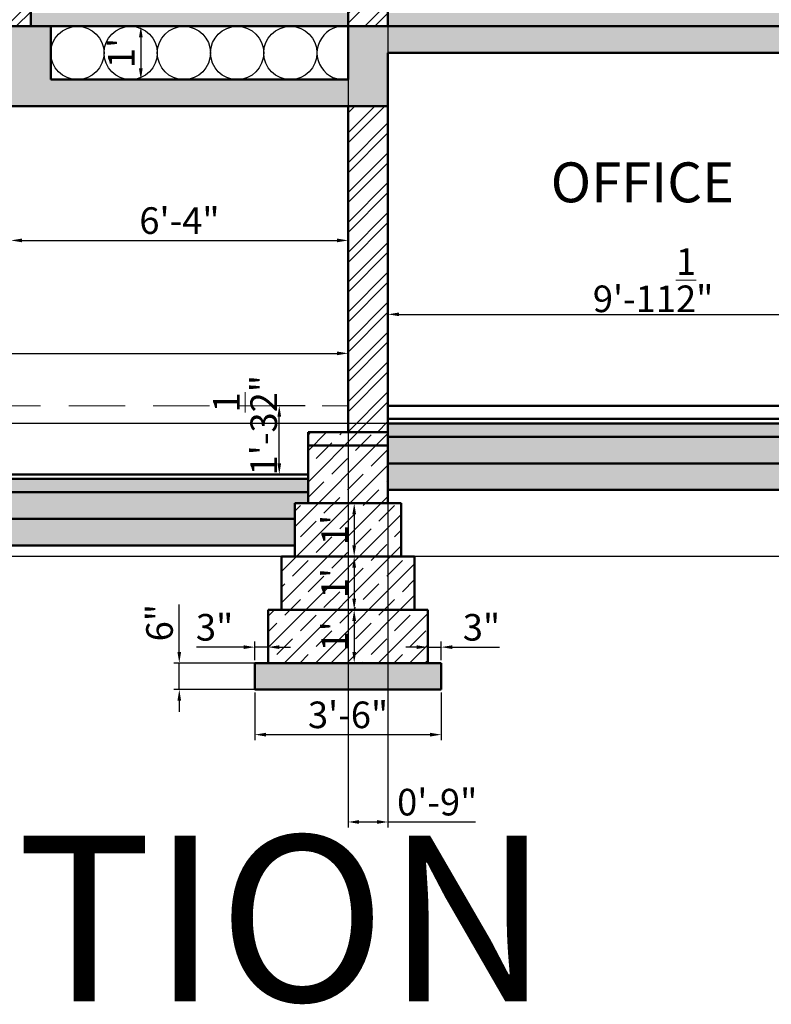
# Model space of a CAD drawing. Units: inches. Extents: x 1615 to 2231, y 1931 to 2519.
# Tile 3 of 6: x 1892 to 2061, y 1931 to 2153. Entities that reach past the tile are written whole.
import ezdxf

# ---------------------------------------------------------------- set-up
doc = ezdxf.new("R2010")
doc.units = ezdxf.units.IN
doc.linetypes.add('DASHED', pattern=[19.05, 12.7, -6.35])
for name, color, linetype, lineweight in [('A-ANNO-DIMS', 2, 'Continuous', 18), ('A-ANNO-TEXT', 7, 'Continuous', 35), ('A-AREA-IDEN', 7, 'Continuous', 25), ('A-SECT', 7, 'Continuous', 50), ('A-SECT-HIDN', 8, 'DASHED', 18), ('A-WALL-PATT', 8, 'Continuous', 13), ('C-TOPO-PATT', 252, 'Continuous', 13), ('S-FNDN', 1, 'Continuous', 50), ('S-FNDN-PATT', 8, 'Continuous', 13), ('S-SLAB', 7, 'Continuous', 25)]:
    doc.layers.add(name, color=color, linetype=linetype, lineweight=lineweight)
doc.styles.get("Standard").update_dxf_attribs({"font": 'arial.ttf'})
doc.dimstyles.new('ISO-25', dxfattribs={"dimtxt": 6, "dimasz": 2.5, "dimexe": 1.25, "dimexo": 0.625, "dimtad": 1, "dimdec": 1, "dimlunit": 4, "dimtxsty": 'Standard', "dimcen": 2.5, "dimadec": 0, "dimazin": 0, "dimtfac": 1, "dimtdec": 1, "dimtmove": 0, "dimatfit": 3, "dimfxl": 1, "dimarcsym": 0})

# ---------------------------------------------------------------- blocks, each defined once
blk = doc.blocks.new('*D9')
at = {"layer": 'A-ANNO-DIMS', "color": 0, "lineweight": -2, "transparency": 16777216}
for p, q in [((1693.37, 2070.69), (1693.37, 2079.07)), ((1695.87, 2077.82), (1963.37, 2077.82)), ((1965.87, 2070.69), (1965.87, 2079.07))]:
    blk.add_line(p, q, dxfattribs=at)
at = {"layer": 'A-ANNO-DIMS', "color": 0, "lineweight": 100, "transparency": 16777216}
for points in [[(1695.87, 2078.24), (1695.87, 2077.4), (1693.37, 2077.82)], [(1963.37, 2078.24), (1963.37, 2077.4), (1965.87, 2077.82)]]:
    blk.add_solid(points, dxfattribs=at)
at = {"layer": 'Defpoints', "color": 0, "lineweight": 100, "transparency": 16777216}
for p in [(1965.87, 2077.82), (1693.37, 2070.06), (1965.87, 2070.06)]:
    blk.add_point(p, dxfattribs=at)
at = {"layer": 'A-ANNO-DIMS', "color": 0, "transparency": 16777216, "insert": (1829.62, 2085.52), "char_height": 6, "attachment_point": 5}
blk.add_mtext('22\'-8{\\H1x;\\S1/2;}"', dxfattribs=at)
blk = doc.blocks.new('*D10')
at = {"layer": 'A-ANNO-DIMS', "color": 0, "lineweight": -2, "transparency": 16777216}
for p, q in [((1956.24, 2066.03), (1949.12, 2066.03)), ((1950.37, 2053.03), (1950.37, 2063.53)), ((1956.24, 2050.53), (1949.12, 2050.53))]:
    blk.add_line(p, q, dxfattribs=at)
at = {"layer": 'A-ANNO-DIMS', "color": 0, "lineweight": 100, "transparency": 16777216}
for points in [[(1949.96, 2063.53), (1950.79, 2063.53), (1950.37, 2066.03)], [(1949.96, 2053.03), (1950.79, 2053.03), (1950.37, 2050.53)]]:
    blk.add_solid(points, dxfattribs=at)
at = {"layer": 'Defpoints', "color": 0, "lineweight": 100, "transparency": 16777216}
for p in [(1950.37, 2066.03), (1956.87, 2066.03), (1956.87, 2050.53)]:
    blk.add_point(p, dxfattribs=at)
at = {"layer": 'A-ANNO-DIMS', "color": 0, "transparency": 16777216, "insert": (1942.67, 2061.63), "char_height": 6, "attachment_point": 5, "rotation": 90}
blk.add_mtext('1\'-3{\\H1x;\\S1/2;}"', dxfattribs=at)
blk = doc.blocks.new('*D17')
at = {"layer": 'A-ANNO-DIMS', "color": 0, "lineweight": -2, "transparency": 16777216}
for p, q in [((1944.87, 2001.4), (1944.87, 1990.63)), ((1986.87, 2001.4), (1986.87, 1990.63)), ((1947.37, 1991.88), (1984.37, 1991.88))]:
    blk.add_line(p, q, dxfattribs=at)
at = {"layer": 'A-ANNO-DIMS', "color": 0, "lineweight": 100, "transparency": 16777216}
for points in [[(1947.37, 1992.3), (1947.37, 1991.46), (1944.87, 1991.88)], [(1984.37, 1992.3), (1984.37, 1991.46), (1986.87, 1991.88)]]:
    blk.add_solid(points, dxfattribs=at)
at = {"layer": 'Defpoints', "color": 0, "lineweight": 100, "transparency": 16777216}
for p in [(1944.87, 2002.03), (1986.87, 2002.03), (1986.87, 1991.88)]:
    blk.add_point(p, dxfattribs=at)
at = {"layer": 'A-ANNO-DIMS', "color": 0, "transparency": 16777216, "insert": (1965.87, 1995.57), "char_height": 6, "attachment_point": 5}
blk.add_mtext('3\'-6"', dxfattribs=at)
blk = doc.blocks.new('*D18')
at = {"layer": 'A-ANNO-DIMS', "color": 0, "lineweight": -2, "transparency": 16777216}
for p, q in [((1983.87, 2008.41), (1983.87, 2012.86)), ((1986.87, 2008.65), (1986.87, 2012.86)), ((1981.37, 2011.61), (1978.87, 2011.61)), ((1983.87, 2011.61), (1986.87, 2011.61)), ((1989.37, 2011.61), (2000.01, 2011.61))]:
    blk.add_line(p, q, dxfattribs=at)
at = {"layer": 'A-ANNO-DIMS', "color": 0, "lineweight": 100, "transparency": 16777216}
for points in [[(1981.37, 2012.02), (1981.37, 2011.19), (1983.87, 2011.61)], [(1989.37, 2012.02), (1989.37, 2011.19), (1986.87, 2011.61)]]:
    blk.add_solid(points, dxfattribs=at)
at = {"layer": 'Defpoints', "color": 0, "lineweight": 100, "transparency": 16777216}
for p in [(1986.87, 2011.61), (1983.87, 2007.79), (1986.87, 2008.03)]:
    blk.add_point(p, dxfattribs=at)
at = {"layer": 'A-ANNO-DIMS', "color": 0, "transparency": 16777216, "insert": (1995.94, 2015.3), "char_height": 6, "attachment_point": 5}
blk.add_mtext('3"', dxfattribs=at)
blk = doc.blocks.new('*D19')
at = {"layer": 'A-ANNO-DIMS', "color": 0, "lineweight": -2, "transparency": 16777216}
for p, q in [((1944.87, 2008.65), (1944.87, 2012.86)), ((1947.87, 2008.65), (1947.87, 2012.86)), ((1942.37, 2011.61), (1931.72, 2011.61)), ((1947.87, 2011.61), (1944.87, 2011.61)), ((1950.37, 2011.61), (1952.87, 2011.61))]:
    blk.add_line(p, q, dxfattribs=at)
at = {"layer": 'A-ANNO-DIMS', "color": 0, "lineweight": 100, "transparency": 16777216}
for points in [[(1942.37, 2012.02), (1942.37, 2011.19), (1944.87, 2011.61)], [(1950.37, 2012.02), (1950.37, 2011.19), (1947.87, 2011.61)]]:
    blk.add_solid(points, dxfattribs=at)
at = {"layer": 'Defpoints', "color": 0, "lineweight": 100, "transparency": 16777216}
for p in [(1944.87, 2011.61), (1944.87, 2008.03), (1947.87, 2008.03)]:
    blk.add_point(p, dxfattribs=at)
at = {"layer": 'A-ANNO-DIMS', "color": 0, "transparency": 16777216, "insert": (1935.79, 2015.3), "char_height": 6, "attachment_point": 5}
blk.add_mtext('3"', dxfattribs=at)
blk = doc.blocks.new('*D20')
at = {"layer": 'A-ANNO-DIMS', "color": 0, "lineweight": -2, "transparency": 16777216}
for p, q in [((1954.49, 2044.03), (1968.51, 2044.03)), ((1967.26, 2041.53), (1967.26, 2034.53)), ((1954.49, 2032.03), (1968.51, 2032.03))]:
    blk.add_line(p, q, dxfattribs=at)
at = {"layer": 'A-ANNO-DIMS', "color": 0, "lineweight": 100, "transparency": 16777216}
for points in [[(1966.84, 2041.53), (1967.67, 2041.53), (1967.26, 2044.03)], [(1966.84, 2034.53), (1967.67, 2034.53), (1967.26, 2032.03)]]:
    blk.add_solid(points, dxfattribs=at)
at = {"layer": 'Defpoints', "color": 0, "lineweight": 100, "transparency": 16777216}
for p in [(1953.87, 2044.03), (1953.87, 2032.03), (1967.26, 2032.03)]:
    blk.add_point(p, dxfattribs=at)
at = {"layer": 'A-ANNO-DIMS', "color": 0, "transparency": 16777216, "insert": (1963.62, 2038.03), "char_height": 6, "attachment_point": 5, "rotation": 90}
blk.add_mtext("1'", dxfattribs=at)
blk = doc.blocks.new('*D21')
at = {"layer": 'A-ANNO-DIMS', "color": 0, "lineweight": -2, "transparency": 16777216}
for p, q in [((1954.49, 2032.03), (1968.51, 2032.03)), ((1967.26, 2029.53), (1967.26, 2022.53)), ((1954.49, 2020.03), (1968.51, 2020.03))]:
    blk.add_line(p, q, dxfattribs=at)
at = {"layer": 'A-ANNO-DIMS', "color": 0, "lineweight": 100, "transparency": 16777216}
for points in [[(1966.84, 2029.53), (1967.67, 2029.53), (1967.26, 2032.03)], [(1966.84, 2022.53), (1967.67, 2022.53), (1967.26, 2020.03)]]:
    blk.add_solid(points, dxfattribs=at)
at = {"layer": 'Defpoints', "color": 0, "lineweight": 100, "transparency": 16777216}
for p in [(1953.87, 2032.03), (1953.87, 2020.03), (1967.26, 2020.03)]:
    blk.add_point(p, dxfattribs=at)
at = {"layer": 'A-ANNO-DIMS', "color": 0, "transparency": 16777216, "insert": (1963.62, 2026.03), "char_height": 6, "attachment_point": 5, "rotation": 90}
blk.add_mtext("1'", dxfattribs=at)
blk = doc.blocks.new('*D22')
at = {"layer": 'A-ANNO-DIMS', "color": 0, "lineweight": -2, "transparency": 16777216}
for p, q in [((1967.88, 2020.03), (1968.51, 2020.03)), ((1967.26, 2017.53), (1967.26, 2010.53)), ((1967.88, 2008.03), (1968.51, 2008.03))]:
    blk.add_line(p, q, dxfattribs=at)
at = {"layer": 'A-ANNO-DIMS', "color": 0, "lineweight": 100, "transparency": 16777216}
for points in [[(1966.84, 2017.53), (1967.67, 2017.53), (1967.26, 2020.03)], [(1966.84, 2010.53), (1967.67, 2010.53), (1967.26, 2008.03)]]:
    blk.add_solid(points, dxfattribs=at)
at = {"layer": 'Defpoints', "color": 0, "lineweight": 100, "transparency": 16777216}
for p in [(1967.26, 2020.03), (1967.26, 2008.03), (1967.26, 2008.03)]:
    blk.add_point(p, dxfattribs=at)
at = {"layer": 'A-ANNO-DIMS', "color": 0, "transparency": 16777216, "insert": (1963.62, 2014.03), "char_height": 6, "attachment_point": 5, "rotation": 90}
blk.add_mtext("1'", dxfattribs=at)
blk = doc.blocks.new('*D25')
at = {"layer": 'A-ANNO-DIMS', "color": 0, "lineweight": -2, "transparency": 16777216}
for p, q in [((1928.24, 2151.53), (1917.92, 2151.53)), ((1919.17, 2149.03), (1919.17, 2142.03)), ((1928.24, 2139.53), (1917.92, 2139.53))]:
    blk.add_line(p, q, dxfattribs=at)
at = {"layer": 'A-ANNO-DIMS', "color": 0, "lineweight": 100, "transparency": 16777216}
for points in [[(1918.75, 2149.03), (1919.58, 2149.03), (1919.17, 2151.53)], [(1918.75, 2142.03), (1919.58, 2142.03), (1919.17, 2139.53)]]:
    blk.add_solid(points, dxfattribs=at)
at = {"layer": 'Defpoints', "color": 0, "lineweight": 100, "transparency": 16777216}
for p in [(1928.87, 2151.53), (1919.17, 2139.53), (1928.87, 2139.53)]:
    blk.add_point(p, dxfattribs=at)
at = {"layer": 'A-ANNO-DIMS', "color": 0, "transparency": 16777216, "insert": (1915.53, 2145.53), "char_height": 6, "attachment_point": 5, "rotation": 90}
blk.add_mtext("1'", dxfattribs=at)
blk = doc.blocks.new('*D26')
at = {"layer": 'A-ANNO-DIMS', "color": 0, "lineweight": -2, "transparency": 16777216}
for p, q in [((1889.87, 2110.4), (1889.87, 2102.03)), ((1965.87, 2110.4), (1965.87, 2102.03)), ((1892.37, 2103.28), (1963.37, 2103.28))]:
    blk.add_line(p, q, dxfattribs=at)
at = {"layer": 'A-ANNO-DIMS', "color": 0, "lineweight": 100, "transparency": 16777216}
for points in [[(1892.37, 2103.7), (1892.37, 2102.86), (1889.87, 2103.28)], [(1963.37, 2103.7), (1963.37, 2102.86), (1965.87, 2103.28)]]:
    blk.add_solid(points, dxfattribs=at)
at = {"layer": 'Defpoints', "color": 0, "lineweight": 100, "transparency": 16777216}
for p in [(1889.87, 2111.03), (1965.87, 2111.03), (1965.87, 2103.28)]:
    blk.add_point(p, dxfattribs=at)
at = {"layer": 'A-ANNO-DIMS', "color": 0, "transparency": 16777216, "insert": (1927.87, 2106.97), "char_height": 6, "attachment_point": 5}
blk.add_mtext('6\'-4"', dxfattribs=at)
blk = doc.blocks.new('*D27')
at = {"layer": 'A-ANNO-DIMS', "color": 0, "lineweight": -2, "transparency": 16777216}
for p, q in [((1974.87, 2077.27), (1974.87, 2087.86)), ((1977.37, 2086.61), (2091.87, 2086.61)), ((2094.37, 2077.27), (2094.37, 2087.86))]:
    blk.add_line(p, q, dxfattribs=at)
at = {"layer": 'A-ANNO-DIMS', "color": 0, "lineweight": 100, "transparency": 16777216}
for points in [[(1977.37, 2087.03), (1977.37, 2086.2), (1974.87, 2086.61)], [(2091.87, 2087.03), (2091.87, 2086.2), (2094.37, 2086.61)]]:
    blk.add_solid(points, dxfattribs=at)
at = {"layer": 'Defpoints', "color": 0, "lineweight": 100, "transparency": 16777216}
for p in [(2094.37, 2086.61), (1974.87, 2076.64), (2094.37, 2076.64)]:
    blk.add_point(p, dxfattribs=at)
at = {"layer": 'A-ANNO-DIMS', "color": 0, "transparency": 16777216, "insert": (2034.62, 2094.31), "char_height": 6, "attachment_point": 5}
blk.add_mtext('9\'-11{\\H1x;\\S1/2;}"', dxfattribs=at)
blk = doc.blocks.new('*D73')
at = {"layer": 'A-ANNO-DIMS', "color": 0, "lineweight": -2, "transparency": 16777216}
for p, q in [((1927.84, 2010.53), (1927.84, 2021.21)), ((1986.24, 2008.03), (1926.59, 2008.03)), ((1927.84, 2002.03), (1927.84, 2008.03)), ((1986.24, 2002.03), (1926.59, 2002.03)), ((1927.84, 1999.53), (1927.84, 1997.03))]:
    blk.add_line(p, q, dxfattribs=at)
at = {"layer": 'A-ANNO-DIMS', "color": 0, "lineweight": 100, "transparency": 16777216}
for points in [[(1927.42, 2010.53), (1928.25, 2010.53), (1927.84, 2008.03)], [(1927.42, 1999.53), (1928.25, 1999.53), (1927.84, 2002.03)]]:
    blk.add_solid(points, dxfattribs=at)
at = {"layer": 'Defpoints', "color": 0, "lineweight": 100, "transparency": 16777216}
for p in [(1927.84, 2008.03), (1986.87, 2008.03), (1986.87, 2002.03)]:
    blk.add_point(p, dxfattribs=at)
at = {"layer": 'A-ANNO-DIMS', "color": 0, "transparency": 16777216, "insert": (1924.15, 2017.12), "char_height": 6, "attachment_point": 5, "rotation": 90}
blk.add_mtext('6"', dxfattribs=at)
blk = doc.blocks.new('*D83')
at = {"layer": 'A-ANNO-DIMS', "color": 0, "lineweight": -2, "transparency": 16777216}
for p, q in [((1965.87, 2420.67), (1965.87, 1970.95)), ((1974.87, 2420.67), (1974.87, 1970.95)), ((1968.37, 1972.2), (1972.37, 1972.2)), ((1974.87, 1972.2), (1994.57, 1972.2))]:
    blk.add_line(p, q, dxfattribs=at)
at = {"layer": 'A-ANNO-DIMS', "color": 0, "lineweight": 100, "transparency": 16777216}
for points in [[(1968.37, 1972.62), (1968.37, 1971.78), (1965.87, 1972.2)], [(1972.37, 1972.62), (1972.37, 1971.78), (1974.87, 1972.2)]]:
    blk.add_solid(points, dxfattribs=at)
at = {"layer": 'Defpoints', "color": 0, "lineweight": 100, "transparency": 16777216}
for p in [(1965.87, 2421.29), (1974.87, 2421.29), (1974.87, 1972.2)]:
    blk.add_point(p, dxfattribs=at)
at = {"layer": 'A-ANNO-DIMS', "color": 0, "transparency": 16777216, "insert": (1985.97, 1975.89), "char_height": 6, "attachment_point": 5}
blk.add_mtext('0\'-9"', dxfattribs=at)
blk = doc.blocks.new('*D88')
at = {"layer": 'A-ANNO-DIMS', "color": 0, "lineweight": -2, "transparency": 16777216}
for p, q in [((2162.74, 2062.03), (1621.79, 2062.03)), ((1623.04, 2059.53), (1623.04, 2034.53)), ((2165.74, 2032.03), (1621.79, 2032.03))]:
    blk.add_line(p, q, dxfattribs=at)
at = {"layer": 'A-ANNO-DIMS', "color": 0, "lineweight": 100, "transparency": 16777216}
for points in [[(1622.62, 2059.53), (1623.46, 2059.53), (1623.04, 2062.03)], [(1622.62, 2034.53), (1623.46, 2034.53), (1623.04, 2032.03)]]:
    blk.add_solid(points, dxfattribs=at)
at = {"layer": 'Defpoints', "color": 0, "lineweight": 100, "transparency": 16777216}
for p in [(2163.37, 2062.03), (1623.04, 2032.03), (2166.37, 2032.03)]:
    blk.add_point(p, dxfattribs=at)
at = {"layer": 'A-ANNO-DIMS', "color": 0, "transparency": 16777216, "insert": (1619.35, 2047.03), "char_height": 6, "attachment_point": 5, "rotation": 90}
blk.add_mtext('2\'-6"', dxfattribs=at)

msp = doc.modelspace()

# ---------------------------------------------------------------- hatches: boundary and pattern name
at = {"layer": 'A-WALL-PATT'}
h = msp.add_hatch(dxfattribs=at)
h.set_pattern_fill('ANSI32', color=256, scale=0.5)
h.paths.add_polyline_path([(1676.87, 2421.53), (1667.87, 2421.53), (1667.87, 2295.53), (1676.87, 2295.53)])
h.paths.add_polyline_path([(1676.87, 2277.53), (1667.87, 2277.53), (1667.87, 2151.53), (1676.87, 2151.53)])
h.paths.add_polyline_path([(1676.87, 2476.53), (1667.87, 2476.53), (1667.87, 2439.53), (1676.87, 2439.53)])
h.paths.add_polyline_path([(1894.37, 2421.29), (1889.87, 2421.29), (1889.87, 2295.53), (1894.37, 2295.53)])
h.paths.add_polyline_path([(1974.87, 2421.29), (1965.87, 2421.29), (1965.87, 2295.53), (1974.87, 2295.53)])
h.paths.add_polyline_path([(2151.37, 2421.29), (2142.37, 2421.29), (2142.37, 2295.53), (2151.37, 2295.53)])
h.paths.add_polyline_path([(2151.37, 2476.53), (2142.37, 2476.53), (2142.37, 2442.53), (2151.37, 2442.53)])
h.paths.add_polyline_path([(1974.87, 2277.53), (1965.87, 2277.53), (1965.87, 2151.53), (1974.87, 2151.53)])
h.paths.add_polyline_path([(1974.87, 2133.53), (1965.87, 2133.53), (1965.87, 2060.03), (1974.87, 2060.03)])
h.paths.add_polyline_path([(2098.87, 2145.53), (2094.37, 2145.53), (2094.37, 2059.03), (2098.87, 2059.03)])
h = msp.add_hatch(dxfattribs=at)
h.set_pattern_fill('DOTS', color=256, scale=0.5)
h.paths.add_polyline_path([(2142.37, 2442.53), (1839.37, 2442.53), (1676.87, 2442.53), (1676.87, 2439.53), (2142.37, 2439.53)])
h.paths.add_polyline_path([(1889.87, 2298.53), (1676.87, 2298.53), (1676.87, 2295.53), (1889.87, 2295.53)])
h.paths.add_polyline_path([(2142.37, 2298.53), (1974.87, 2298.53), (1974.87, 2295.53), (2142.37, 2295.53)])
h.paths.add_polyline_path([(1889.87, 2154.53), (1676.87, 2154.53), (1676.87, 2151.53), (1889.87, 2151.53)])
h.paths.add_polyline_path([(1965.87, 2154.53), (1894.37, 2154.53), (1894.37, 2151.53), (1965.87, 2151.53)])
h.paths.add_polyline_path([(2142.37, 2154.53), (1974.87, 2154.53), (1974.87, 2151.53), (2142.37, 2151.53)])
h.paths.add_polyline_path([(2094.37, 2062.03), (1974.87, 2062.03), (1974.87, 2059.03), (2094.37, 2059.03)])
h.paths.add_polyline_path([(2142.37, 2062.03), (2098.87, 2062.03), (2098.87, 2059.03), (2142.37, 2059.03)])
h.paths.add_polyline_path([(1956.87, 2049.53), (1693.37, 2049.53), (1693.37, 2046.53), (1956.87, 2046.53)])
h = msp.add_hatch(dxfattribs=at)
h.set_pattern_fill('AR-CONC', color=256, scale=0.1)
h.paths.add_polyline_path([(1898.87, 2151.53), (1667.87, 2151.53), (1667.87, 2145.53), (1679.87, 2145.53), (1682.87, 2145.53), (1889.87, 2145.53), (1889.87, 2133.53), (1974.87, 2133.53), (1974.87, 2145.53), (2142.37, 2145.53), (2142.37, 2133.53), (2157.37, 2133.53), (2157.37, 2151.53), (2155.87, 2151.53), (2151.37, 2151.53), (1965.87, 2151.53), (1965.87, 2139.53), (1898.87, 2139.53)])
h.paths.add_polyline_path([(1898.87, 2295.53), (1667.87, 2295.53), (1667.87, 2277.53), (1676.87, 2277.53), (1676.87, 2289.53), (1889.87, 2289.53), (1889.87, 2277.53), (1974.87, 2277.53), (1974.87, 2289.53), (2142.37, 2289.53), (2142.37, 2277.53), (2151.37, 2277.53), (2151.37, 2295.53), (1965.87, 2295.53), (1965.87, 2283.53), (1898.87, 2283.53)])
h.paths.add_polyline_path([(2142.37, 2439.53), (1676.87, 2439.53), (1667.87, 2439.53), (1667.87, 2421.53), (1676.87, 2421.53), (1676.87, 2433.53), (1889.87, 2433.53), (1889.87, 2421.29), (1898.87, 2421.29), (1898.87, 2433.53), (1965.87, 2433.53), (1965.87, 2421.29), (1974.87, 2421.29), (1974.87, 2433.53), (2142.37, 2433.53)])
h = msp.add_hatch(dxfattribs=at)
h.set_pattern_fill('ANSI32', color=256, scale=0.5)
h.paths.add_polyline_path([(2151.37, 2277.53), (2142.37, 2277.53), (2142.37, 2151.53), (2151.37, 2151.53)])
h.paths.add_polyline_path([(1894.37, 2277.53), (1889.87, 2277.53), (1889.87, 2151.53), (1894.37, 2151.53)])
h = msp.add_hatch(dxfattribs=at)
h.set_pattern_fill('JIS_STN_1E', color=256, scale=5)
h.paths.add_polyline_path([(1688.87, 2100.53), (1655.87, 2100.53), (1655.87, 2088.53), (1688.87, 2088.53)])
h.paths.add_polyline_path([(1685.87, 2112.53), (1658.87, 2112.53), (1658.87, 2100.53), (1685.87, 2100.53)])
h.paths.add_polyline_path([(1682.87, 2139.53), (1661.87, 2139.53), (1661.87, 2112.53), (1682.87, 2112.53)])
h.paths.add_polyline_path([(1688.87, 2088.53), (1655.87, 2088.53), (1652.87, 2088.53), (1652.87, 2082.53), (1688.87, 2082.53)])
h.paths.add_polyline_path([(1682.87, 2145.53), (1679.87, 2145.53), (1676.87, 2145.53), (1661.87, 2145.53), (1661.87, 2139.53), (1682.87, 2139.53)])
h.paths.add_polyline_path([(1974.87, 2057.03), (1956.87, 2057.03), (1956.87, 2044.03), (1974.87, 2044.03)])
h.paths.add_polyline_path([(1974.87, 2060.03), (1956.87, 2060.03), (1956.87, 2057.03), (1974.87, 2057.03)])
h.paths.add_polyline_path([(1980.87, 2032.03), (1950.87, 2032.03), (1950.87, 2020.03), (1980.87, 2020.03)])
h.paths.add_polyline_path([(1977.87, 2044.03), (1953.87, 2044.03), (1953.87, 2032.03), (1977.87, 2032.03)])
h.paths.add_polyline_path([(1983.87, 2020.03), (1947.87, 2020.03), (1947.87, 2008.03), (1983.87, 2008.03)])
h.paths.add_polyline_path([(2104.12, 2056.03), (2089.12, 2056.03), (2089.12, 2032.03), (2104.12, 2032.03)])
h.paths.add_polyline_path([(2104.12, 2059.03), (2089.12, 2059.03), (2089.12, 2056.03), (2104.12, 2056.03)])
h.paths.add_polyline_path([(2105.62, 2032.03), (2087.62, 2032.03), (2087.62, 2020.03), (2105.62, 2020.03)])
h.paths.add_polyline_path([(2107.12, 2020.03), (2086.12, 2020.03), (2086.12, 2008.03), (2107.12, 2008.03)])
h.paths.add_polyline_path([(2169.37, 2032.03), (2139.37, 2032.03), (2139.37, 2020.03), (2169.37, 2020.03)])
h.paths.add_polyline_path([(2172.37, 2020.03), (2136.37, 2020.03), (2136.37, 2008.03), (2172.37, 2008.03)])
h.paths.add_polyline_path([(2166.37, 2062.03), (2163.37, 2062.03), (2163.37, 2089.03), (2160.37, 2089.03), (2160.37, 2112.53), (2157.37, 2112.53), (2157.37, 2133.53), (2142.37, 2133.53), (2142.37, 2032.03), (2166.37, 2032.03)])
at = {"layer": 'C-TOPO-PATT'}
h = msp.add_hatch(dxfattribs=at)
h.set_pattern_fill('GRAVEL', color=256, scale=0.5, angle=27)
h.paths.add_polyline_path([(1956.87, 2046.53), (1693.37, 2046.53), (1693.37, 2040.53), (1953.87, 2040.53), (1953.87, 2044.03), (1956.87, 2044.03)])
h.paths.add_polyline_path([(2089.12, 2059.03), (1974.87, 2059.03), (1974.87, 2053.03), (2089.12, 2053.03)])
h.paths.add_polyline_path([(2142.37, 2059.03), (2104.12, 2059.03), (2104.12, 2053.03), (2142.37, 2053.03)])
h.paths.add_polyline_path([(2195.62, 2124.53), (2157.37, 2124.53), (2157.37, 2118.53), (2195.62, 2118.53)])
h = msp.add_hatch(dxfattribs=at)
h.set_pattern_fill('EARTH', color=256, angle=27)
h.paths.add_polyline_path([(1953.87, 2040.53), (1693.37, 2040.53), (1693.37, 2034.53), (1696.37, 2034.53), (1953.87, 2034.53)])
h.paths.add_polyline_path([(2089.12, 2053.03), (1974.87, 2053.03), (1974.87, 2047.03), (2089.12, 2047.03)])
h.paths.add_polyline_path([(2142.37, 2053.03), (2104.12, 2053.03), (2104.12, 2047.03), (2142.37, 2047.03)])
at = {"layer": 'S-FNDN-PATT'}
h = msp.add_hatch(dxfattribs=at)
h.set_pattern_fill('AR-CONC', color=256, scale=0.1)
h.paths.add_polyline_path([(1702.37, 2010.53), (1667.87, 2010.53), (1667.87, 2004.53), (1702.37, 2004.53)])
h.paths.add_polyline_path([(1986.87, 2008.03), (1944.87, 2008.03), (1944.87, 2002.03), (1986.87, 2002.03)])
h.paths.add_polyline_path([(2108.62, 2008.03), (2084.62, 2008.03), (2084.62, 2002.03), (2108.62, 2002.03)])
h.paths.add_polyline_path([(2175.37, 2008.03), (2133.37, 2008.03), (2133.37, 2002.03), (2175.37, 2002.03)])

# ---------------------------------------------------------------- linework, layer by layer
at = {"layer": 'A-SECT'}
for p, q in [((1974.87, 2289.53), (1974.87, 2151.53)), ((1894.37, 2277.53), (1894.37, 2151.53)), ((1965.87, 2277.53), (1965.87, 2139.53)), ((1667.87, 2151.53), (2151.37, 2151.53)), ((1898.87, 2151.53), (1898.87, 2139.53)), ((1974.87, 2145.53), (2142.37, 2145.53)), ((1974.87, 2145.53), (1974.87, 2044.03)), ((1898.87, 2139.53), (1965.87, 2139.53)), ((1889.87, 2133.53), (1974.87, 2133.53)), ((1965.87, 2133.53), (1965.87, 2060.03)), ((1974.87, 2063.03), (2094.37, 2063.03)), ((1974.87, 2062.03), (2094.37, 2062.03)), ((1974.87, 2059.03), (2142.37, 2059.03)), ((1974.87, 2053.03), (2089.12, 2053.03)), ((1693.37, 2050.53), (1956.87, 2050.53)), ((1693.37, 2049.53), (1956.87, 2049.53)), ((1693.37, 2046.53), (1956.87, 2046.53)), ((1974.87, 2047.03), (2089.12, 2047.03)), ((1693.37, 2040.53), (1953.87, 2040.53))]:
    msp.add_line(p, q, dxfattribs=at)
at = {"layer": 'A-SECT-HIDN'}
msp.add_line((1693.37, 2066.03), (1965.87, 2066.03), dxfattribs=at)
at = {"layer": 'S-FNDN'}
for p, q in [((1974.87, 2066.03), (2094.37, 2066.03)), ((1956.87, 2060.03), (1956.87, 2044.03)), ((1956.87, 2060.03), (1974.87, 2060.03)), ((1956.87, 2057.03), (1974.87, 2057.03)), ((1953.87, 2044.03), (1953.87, 2032.03)), ((1953.87, 2044.03), (1977.87, 2044.03)), ((1977.87, 2044.03), (1977.87, 2032.03)), ((1696.37, 2034.53), (1953.87, 2034.53)), ((1950.87, 2032.03), (1980.87, 2032.03)), ((1950.87, 2032.03), (1950.87, 2020.03)), ((1980.87, 2032.03), (1980.87, 2020.03)), ((1947.87, 2020.03), (1983.87, 2020.03)), ((1947.87, 2020.03), (1947.87, 2008.03)), ((1983.87, 2020.03), (1983.87, 2008.03)), ((1944.87, 2008.03), (1986.87, 2008.03)), ((1944.87, 2002.03), (1944.87, 2008.03)), ((1986.87, 2008.03), (1986.87, 2002.03)), ((1986.87, 2002.03), (1944.87, 2002.03))]:
    msp.add_line(p, q, dxfattribs=at)
at = {"layer": 'S-SLAB'}
for centre in [(1904.87, 2145.53), (1916.87, 2145.53), (1928.87, 2145.53), (1940.87, 2145.53), (1952.87, 2145.53)]:
    msp.add_circle(centre, 6, dxfattribs=at)
msp.add_arc((1964.87, 2145.53), 6, 80.4059, 279.5941, dxfattribs=at)

# ---------------------------------------------------------------- texts
at = {"layer": 'A-ANNO-TEXT'}
msp.add_text('SECTION', height=37.358, dxfattribs=at).set_placement((1798.24, 1931.77))
at = {"layer": 'A-AREA-IDEN', "insert": (2011.55, 2120.86), "char_height": 9, "attachment_point": 1}
msp.add_mtext_dynamic_manual_height_columns('OFFICE', width=2.6039, gutter_width=12.5, heights=[0], dxfattribs=at)

# ---------------------------------------------------------------- dimensions: what is measured, and where the dimension line sits
at = {"layer": 'A-ANNO-DIMS'}
for base, p1, p2, override, picture, middle in [((1974.87, 1972.2), (1965.87, 2421.29), (1974.87, 2421.29), {"dimdec": 1, "dimlfac": 1, "dimrnd": 0, "dimzin": 1, "dimdsep": 46, "dimlunit": 4, "dimfrac": 2}, '*D83', (1985.97, 1975.89)), ((1965.87, 2103.28), (1889.87, 2111.03), (1965.87, 2111.03), {"dimclrd": 0, "dimclre": 0, "dimclrt": 0}, '*D26', (1927.87, 2106.97)), ((2094.37, 2086.61), (1974.87, 2076.64), (2094.37, 2076.64), {"dimclrd": 0, "dimclre": 0, "dimclrt": 0}, '*D27', (2034.62, 2094.31)), ((1965.87, 2077.82), (1693.37, 2070.06), (1965.87, 2070.06), {"dimclrd": 0, "dimclre": 0, "dimclrt": 0}, '*D9', (1829.62, 2085.52)), ((1944.87, 2011.61), (1947.87, 2008.03), (1944.87, 2008.03), {"dimclrd": 0, "dimclre": 0, "dimclrt": 0}, '*D19', (1935.79, 2015.3)), ((1986.87, 2011.61), (1983.87, 2007.79), (1986.87, 2008.03), {"dimclrd": 0, "dimclre": 0, "dimclrt": 0}, '*D18', (1995.94, 2015.3)), ((1986.87, 1991.88), (1944.87, 2002.03), (1986.87, 2002.03), {"dimclrd": 0, "dimclre": 0, "dimclrt": 0}, '*D17', (1965.87, 1995.57))]:
    dim = msp.add_linear_dim(base=base, p1=p1, p2=p2, dimstyle='ISO-25', override=override, dxfattribs=at)
    dim.commit()
    dim.dimension.update_dxf_attribs({"geometry": picture, "text_midpoint": middle})
for base, p1, p2, override, picture, middle in [((1919.17, 2139.53), (1928.87, 2151.53), (1928.87, 2139.53), {"dimclrd": 0, "dimclre": 0, "dimclrt": 0}, '*D25', (1915.53, 2145.53)), ((1623.04, 2032.03), (2163.37, 2062.03), (2166.37, 2032.03), {"dimdec": 1, "dimlfac": 1, "dimrnd": 0, "dimzin": 1, "dimdsep": 46, "dimlunit": 4, "dimfrac": 2}, '*D88', (1619.35, 2047.03)), ((1967.26, 2032.03), (1953.87, 2044.03), (1953.87, 2032.03), {"dimclrd": 0, "dimclre": 0, "dimclrt": 0}, '*D20', (1963.62, 2038.03)), ((1967.26, 2020.03), (1953.87, 2032.03), (1953.87, 2020.03), {"dimclrd": 0, "dimclre": 0, "dimclrt": 0}, '*D21', (1963.62, 2026.03)), ((1927.84, 2008.03), (1986.87, 2002.03), (1986.87, 2008.03), {"dimclrd": 0, "dimclre": 0, "dimclrt": 0}, '*D73', (1924.15, 2017.12)), ((1967.26, 2008.03), (1967.26, 2020.03), (1967.26, 2008.03), {"dimclrd": 0, "dimclre": 0, "dimclrt": 0}, '*D22', (1963.62, 2014.03))]:
    dim = msp.add_linear_dim(base=base, p1=p1, p2=p2, angle=90, dimstyle='ISO-25', override=override, dxfattribs=at)
    dim.commit()
    dim.dimension.update_dxf_attribs({"geometry": picture, "text_midpoint": middle})
dim = msp.add_linear_dim(base=(1950.37, 2066.03), p1=(1956.87, 2050.53), p2=(1956.87, 2066.03), angle=90, dimstyle='ISO-25', override={"dimclrd": 0, "dimclre": 0, "dimclrt": 0}, dxfattribs=at)
dim.commit()
dim.dimension.update_dxf_attribs({"geometry": '*D10', "text_midpoint": (1950.37, 2061.63), "dimtype": 160})

doc.saveas('drawing.dxf')
